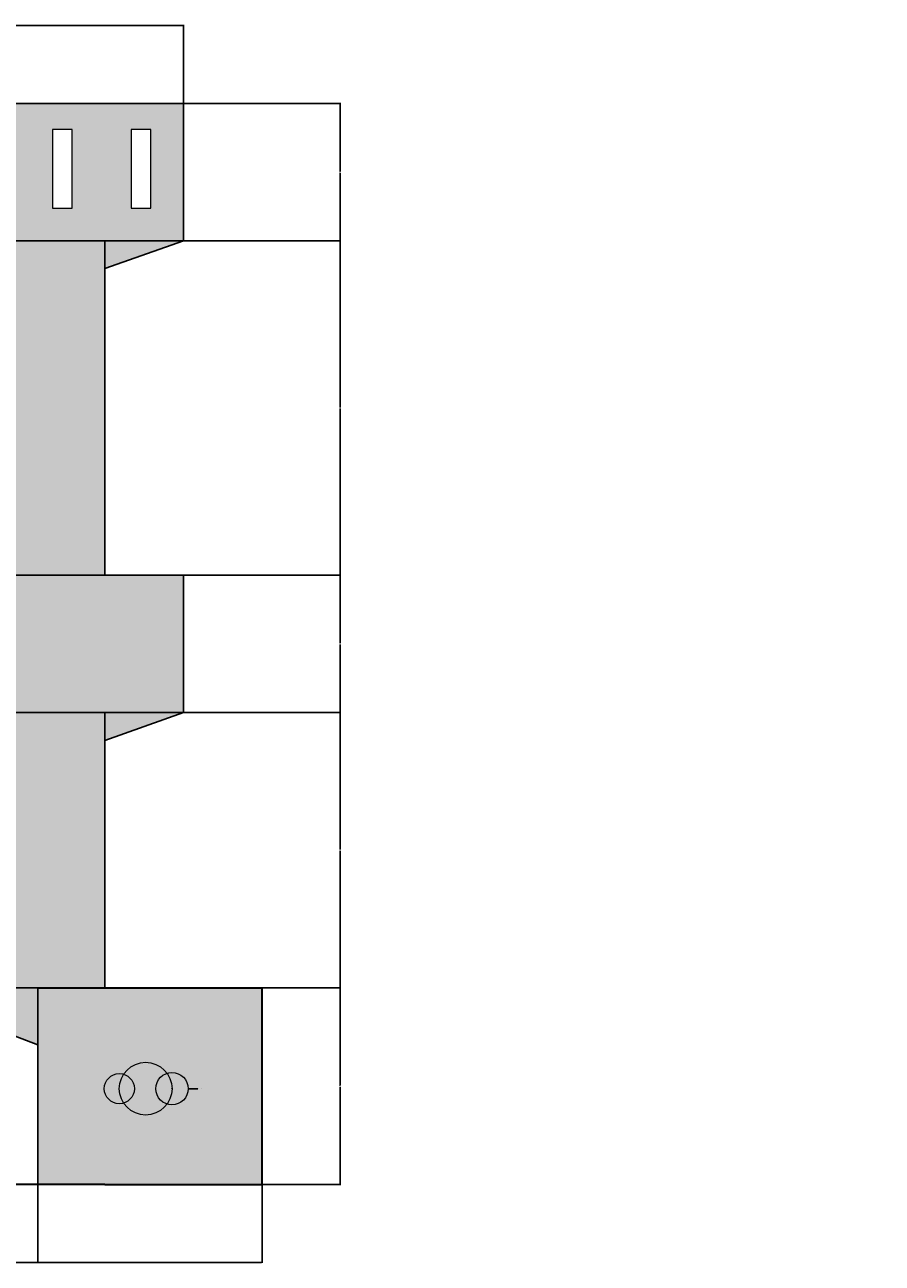
# Model space of a CAD drawing. Units: inches. Extents: x -43 to 1296, y -568 to 542.
# Tile 7 of 14: x 364 to 626, y 164 to 542. Entities that reach past the tile are written whole.
import ezdxf

# ---------------------------------------------------------------- set-up
doc = ezdxf.new("R2010")
doc.units = ezdxf.units.IN
doc.header["$MEASUREMENT"] = 0
for name, color, linetype, lineweight in [('A-ANNO-DIMS', 2, 'Continuous', 18), ('A-ELEV', 7, 'Continuous', 25), ('A-ELEV-TRIM', 7, 'Continuous', 18), ('A-ELEV-TRIM-PATT', 4, 'Continuous', 13), ('A-SITE-GATE', 7, 'Continuous', 25), ('A-SITE-WALL', 7, 'Continuous', 30), ('A-SITE-WALL-PATT', 142, 'Continuous', 13)]:
    doc.layers.add(name, color=color, linetype=linetype, lineweight=lineweight)
for name, color, linetype, lineweight, true_color in [('A-ELEV-BAND-PATT', 30, 'Continuous', 13, 0xf8991e), ('A-ELEV-WALL-PATT', 31, 'Continuous', 13, 0xfecc66), ('A-ROOF-PATT', 217, 'Continuous', 13, 0x93278f)]:
    doc.layers.add(name, color=color, linetype=linetype, lineweight=lineweight, true_color=true_color)
doc.styles.get("Standard").update_dxf_attribs({"font": 'arial.ttf'})
doc.dimstyles.get("Standard").update_dxf_attribs({"dimtxt": 0.18, "dimasz": 0.18, "dimexe": 0.18, "dimexo": 0.0625, "dimgap": 0.09, "dimtad": 0, "dimtih": 1, "dimtoh": 1, "dimdec": 0, "dimzin": 0, "dimdsep": 46, "dimlunit": 3, "dimtxsty": 'Standard', "dimcen": 0.09, "dimadec": 0, "dimazin": 0, "dimtfac": 1, "dimtdec": 0, "dimtofl": 0, "dimtmove": 0, "dimatfit": 3, "dimfxl": 1, "dimtolj": 1, "dimtzin": 0, "dimarcsym": 0})

# ---------------------------------------------------------------- blocks, each defined once
blk = doc.blocks.new('*U5')
for p, q in [((-3, 12), (-3, -12)), ((3, 12), (-3, 12)), ((3, -12), (3, 12)), ((-3, -12), (3, -12))]:
    blk.add_line(p, q)
blk = doc.blocks.new('*U6')
at = {"layer": 'A-ELEV-TRIM', "color": 0, "linetype": 'ByBlock', "lineweight": -2, "transparency": 16777216}
for p in [(0, 0), (24, 0), (48, 0), (72, 0), (96, 0), (120, 0), (144, 0), (168, 0), (192, 0), (216, 0), (240, 0), (264, 0), (288, 0), (312, 0), (336, 0), (360, 0), (384, 0)]:
    blk.add_blockref('*U5', p, dxfattribs=at)
blk = doc.blocks.new('*D60')
at = {"layer": 'A-ANNO-DIMS', "color": 0, "lineweight": -2, "transparency": 16777216}
for p, q in [((-19.16, 188.23), (-19.16, 164.31)), ((436.84, 188.23), (436.84, 164.31)), ((-18.98, 164.49), (208.44, 164.49)), ((436.66, 164.49), (209.24, 164.49))]:
    blk.add_line(p, q, dxfattribs=at)
at = {"layer": 'A-ANNO-DIMS', "color": 0, "transparency": 16777216}
for points in [[(-18.98, 164.52), (-18.98, 164.46), (-19.16, 164.49)], [(436.66, 164.52), (436.66, 164.46), (436.84, 164.49)]]:
    blk.add_solid(points, dxfattribs=at)
at = {"layer": 'Defpoints', "color": 0, "transparency": 16777216}
for p in [(-19.16, 188.29), (436.84, 188.29), (436.84, 164.49)]:
    blk.add_point(p, dxfattribs=at)
at = {"layer": 'A-ANNO-DIMS', "color": 0, "transparency": 16777216, "insert": (208.84, 164.49), "char_height": 0.18, "attachment_point": 5}
blk.add_mtext('\\A1;38\'-0"', dxfattribs=at)
blk = doc.blocks.new('*D62')
at = {"layer": 'A-ANNO-DIMS', "color": 0, "lineweight": -2, "transparency": 16777216}
for p, q in [((436.91, 248.29), (460.82, 248.29)), ((460.64, 248.11), (460.64, 218.47)), ((460.64, 188.47), (460.64, 218.11)), ((436.91, 188.29), (460.82, 188.29))]:
    blk.add_line(p, q, dxfattribs=at)
at = {"layer": 'A-ANNO-DIMS', "color": 0, "transparency": 16777216}
for points in [[(460.61, 248.11), (460.67, 248.11), (460.64, 248.29)], [(460.61, 188.47), (460.67, 188.47), (460.64, 188.29)]]:
    blk.add_solid(points, dxfattribs=at)
at = {"layer": 'Defpoints', "color": 0, "transparency": 16777216}
for p in [(436.84, 248.29), (460.64, 248.29), (436.84, 188.29)]:
    blk.add_point(p, dxfattribs=at)
at = {"layer": 'A-ANNO-DIMS', "color": 0, "transparency": 16777216, "insert": (460.64, 218.29), "char_height": 0.18, "attachment_point": 5}
blk.add_mtext('\\A1;5\'-0"', dxfattribs=at)
blk = doc.blocks.new('*D63')
at = {"layer": 'A-ANNO-DIMS', "color": 0, "lineweight": -2, "transparency": 16777216}
for p, q in [((412.91, 332.29), (460.82, 332.29)), ((460.64, 332.11), (460.64, 290.47)), ((460.64, 248.47), (460.64, 290.11)), ((436.91, 248.29), (460.82, 248.29))]:
    blk.add_line(p, q, dxfattribs=at)
at = {"layer": 'A-ANNO-DIMS', "color": 0, "transparency": 16777216}
for points in [[(460.61, 332.11), (460.67, 332.11), (460.64, 332.29)], [(460.61, 248.47), (460.67, 248.47), (460.64, 248.29)]]:
    blk.add_solid(points, dxfattribs=at)
at = {"layer": 'Defpoints', "color": 0, "transparency": 16777216}
for p in [(412.84, 332.29), (460.64, 332.29), (436.84, 248.29)]:
    blk.add_point(p, dxfattribs=at)
at = {"layer": 'A-ANNO-DIMS', "color": 0, "transparency": 16777216, "insert": (460.64, 290.29), "char_height": 0.18, "attachment_point": 5}
blk.add_mtext('\\A1;7\'-0"', dxfattribs=at)
blk = doc.blocks.new('*D64')
at = {"layer": 'A-ANNO-DIMS', "color": 0, "lineweight": -2, "transparency": 16777216}
for p, q in [((412.91, 374.29), (460.82, 374.29)), ((460.64, 374.11), (460.64, 353.47)), ((460.64, 332.47), (460.64, 353.11)), ((412.91, 332.29), (460.82, 332.29))]:
    blk.add_line(p, q, dxfattribs=at)
at = {"layer": 'A-ANNO-DIMS', "color": 0, "transparency": 16777216}
for points in [[(460.61, 374.11), (460.67, 374.11), (460.64, 374.29)], [(460.61, 332.47), (460.67, 332.47), (460.64, 332.29)]]:
    blk.add_solid(points, dxfattribs=at)
at = {"layer": 'Defpoints', "color": 0, "transparency": 16777216}
for p in [(412.84, 374.29), (460.64, 374.29), (412.84, 332.29)]:
    blk.add_point(p, dxfattribs=at)
at = {"layer": 'A-ANNO-DIMS', "color": 0, "transparency": 16777216, "insert": (460.64, 353.29), "char_height": 0.18, "attachment_point": 5}
blk.add_mtext('\\A1;3\'-6"', dxfattribs=at)
blk = doc.blocks.new('*D65')
at = {"layer": 'A-ANNO-DIMS', "color": 0, "lineweight": -2, "transparency": 16777216}
for p, q in [((412.91, 476.29), (460.82, 476.29)), ((460.64, 476.11), (460.64, 425.47)), ((460.64, 374.47), (460.64, 425.11)), ((412.91, 374.29), (460.82, 374.29))]:
    blk.add_line(p, q, dxfattribs=at)
at = {"layer": 'A-ANNO-DIMS', "color": 0, "transparency": 16777216}
for points in [[(460.61, 476.11), (460.67, 476.11), (460.64, 476.29)], [(460.61, 374.47), (460.67, 374.47), (460.64, 374.29)]]:
    blk.add_solid(points, dxfattribs=at)
at = {"layer": 'Defpoints', "color": 0, "transparency": 16777216}
for p in [(412.84, 476.29), (460.64, 476.29), (412.84, 374.29)]:
    blk.add_point(p, dxfattribs=at)
at = {"layer": 'A-ANNO-DIMS', "color": 0, "transparency": 16777216, "insert": (460.64, 425.29), "char_height": 0.18, "attachment_point": 5}
blk.add_mtext('\\A1;8\'-6"', dxfattribs=at)
blk = doc.blocks.new('*D66')
at = {"layer": 'A-ANNO-DIMS', "color": 0, "lineweight": -2, "transparency": 16777216}
for p, q in [((412.91, 518.29), (460.82, 518.29)), ((460.64, 518.11), (460.64, 497.47)), ((460.64, 476.47), (460.64, 497.11)), ((412.91, 476.29), (460.82, 476.29))]:
    blk.add_line(p, q, dxfattribs=at)
at = {"layer": 'A-ANNO-DIMS', "color": 0, "transparency": 16777216}
for points in [[(460.61, 518.11), (460.67, 518.11), (460.64, 518.29)], [(460.61, 476.47), (460.67, 476.47), (460.64, 476.29)]]:
    blk.add_solid(points, dxfattribs=at)
at = {"layer": 'Defpoints', "color": 0, "transparency": 16777216}
for p in [(412.84, 518.29), (460.64, 518.29), (412.84, 476.29)]:
    blk.add_point(p, dxfattribs=at)
at = {"layer": 'A-ANNO-DIMS', "color": 0, "transparency": 16777216, "insert": (460.64, 497.29), "char_height": 0.18, "attachment_point": 5}
blk.add_mtext('\\A1;3\'-6"', dxfattribs=at)
blk = doc.blocks.new('*D67')
at = {"layer": 'A-ANNO-DIMS', "color": 0, "lineweight": -2, "transparency": 16777216}
for p, q in [((277.84, 188.23), (277.84, 164.31)), ((368.43, 188.23), (368.43, 164.31)), ((278.02, 164.49), (322.6, 164.49)), ((368.25, 164.49), (323.68, 164.49))]:
    blk.add_line(p, q, dxfattribs=at)
at = {"layer": 'A-ANNO-DIMS', "color": 0, "transparency": 16777216}
for points in [[(278.02, 164.52), (278.02, 164.46), (277.84, 164.49)], [(368.25, 164.52), (368.25, 164.46), (368.43, 164.49)]]:
    blk.add_solid(points, dxfattribs=at)
at = {"layer": 'Defpoints', "color": 0, "transparency": 16777216}
for p in [(277.84, 188.29), (368.43, 188.29), (368.43, 164.49)]:
    blk.add_point(p, dxfattribs=at)
at = {"layer": 'A-ANNO-DIMS', "color": 0, "transparency": 16777216, "insert": (323.14, 164.49), "char_height": 0.18, "attachment_point": 5}
blk.add_mtext('\\A1;7\'-6 1/2"', dxfattribs=at)
blk = doc.blocks.new('*D69')
at = {"layer": 'A-ANNO-DIMS', "color": 0, "lineweight": -2, "transparency": 16777216}
for p, q in [((323.2, 248.29), (460.82, 248.29)), ((460.64, 248.11), (460.64, 218.47)), ((460.64, 188.47), (460.64, 218.11)), ((368.5, 188.29), (460.82, 188.29))]:
    blk.add_line(p, q, dxfattribs=at)
at = {"layer": 'A-ANNO-DIMS', "color": 0, "transparency": 16777216}
for points in [[(460.61, 248.11), (460.67, 248.11), (460.64, 248.29)], [(460.61, 188.47), (460.67, 188.47), (460.64, 188.29)]]:
    blk.add_solid(points, dxfattribs=at)
at = {"layer": 'Defpoints', "color": 0, "transparency": 16777216}
for p in [(323.14, 248.29), (368.43, 188.29), (460.64, 188.29)]:
    blk.add_point(p, dxfattribs=at)
at = {"layer": 'A-ANNO-DIMS', "color": 0, "transparency": 16777216, "insert": (460.64, 218.29), "char_height": 0.18, "attachment_point": 5}
blk.add_mtext('\\A1;5\'-0"', dxfattribs=at)
blk = doc.blocks.new('*D72')
at = {"layer": 'A-ANNO-DIMS', "color": 0, "lineweight": -2, "transparency": 16777216}
for p, q in [((368.43, 188.23), (368.43, 164.31)), ((436.84, 188.23), (436.84, 164.31)), ((368.61, 164.49), (402.1, 164.49)), ((436.66, 164.49), (403.18, 164.49))]:
    blk.add_line(p, q, dxfattribs=at)
at = {"layer": 'A-ANNO-DIMS', "color": 0, "transparency": 16777216}
for points in [[(368.61, 164.52), (368.61, 164.46), (368.43, 164.49)], [(436.66, 164.52), (436.66, 164.46), (436.84, 164.49)]]:
    blk.add_solid(points, dxfattribs=at)
at = {"layer": 'Defpoints', "color": 0, "transparency": 16777216}
for p in [(368.43, 188.29), (436.84, 188.29), (436.84, 164.49)]:
    blk.add_point(p, dxfattribs=at)
at = {"layer": 'A-ANNO-DIMS', "color": 0, "transparency": 16777216, "insert": (402.64, 164.49), "char_height": 0.18, "attachment_point": 5}
blk.add_mtext('\\A1;5\'-8 1/2"', dxfattribs=at)
blk = doc.blocks.new('*D73')
at = {"layer": 'A-ANNO-DIMS', "color": 0, "lineweight": -2, "transparency": 16777216}
for p, q in [((4.84, 518.35), (4.84, 542.27)), ((5.02, 542.09), (208.44, 542.09)), ((412.66, 542.09), (209.24, 542.09)), ((412.84, 518.35), (412.84, 542.27))]:
    blk.add_line(p, q, dxfattribs=at)
at = {"layer": 'A-ANNO-DIMS', "color": 0, "transparency": 16777216}
for points in [[(5.02, 542.12), (5.02, 542.06), (4.84, 542.09)], [(412.66, 542.12), (412.66, 542.06), (412.84, 542.09)]]:
    blk.add_solid(points, dxfattribs=at)
at = {"layer": 'Defpoints', "color": 0, "transparency": 16777216}
for p in [(412.84, 542.09), (4.84, 518.29), (412.84, 518.29)]:
    blk.add_point(p, dxfattribs=at)
at = {"layer": 'A-ANNO-DIMS', "color": 0, "transparency": 16777216, "insert": (208.84, 542.09), "char_height": 0.18, "attachment_point": 5}
blk.add_mtext('\\A1;34\'-0"', dxfattribs=at)
blk = doc.blocks.new('*D100')
at = {"layer": 'A-ANNO-DIMS', "color": 0, "lineweight": -2, "transparency": 16777216}
for p, q in [((409.23, 217.51), (409.41, 217.51)), ((409.32, 217.42), (409.32, 217.6)), ((417.2, 217.51), (414.42, 217.51))]:
    blk.add_line(p, q, dxfattribs=at)
at = {"layer": 'A-ANNO-DIMS', "color": 0, "transparency": 16777216}
blk.add_solid([(414.42, 217.54), (414.42, 217.48), (414.24, 217.51)], dxfattribs=at)
at = {"layer": 'Defpoints', "color": 0, "transparency": 16777216}
for p in [(404.4, 217.51), (414.24, 217.51)]:
    blk.add_point(p, dxfattribs=at)
at = {"layer": 'A-ANNO-DIMS', "color": 0, "transparency": 16777216, "insert": (417.88, 217.51), "char_height": 0.18, "attachment_point": 5}
blk.add_mtext('\\A1;3X ∅0\'-10"', dxfattribs=at)

msp = doc.modelspace()

# ---------------------------------------------------------------- hatches: boundary and pattern name
at = {"layer": 'A-ELEV-BAND-PATT'}
h = msp.add_hatch(color=256, dxfattribs=at)
h.dxf.hatch_style = 1
h.paths.add_polyline_path([(28.84, 332.29), (4.84, 332.29), (28.84, 320)])
h.paths.add_polyline_path([(412.84, 332.29), (388.84, 332.29), (388.84, 323.84)])
h.paths.add_polyline_path([(1184.13, 416.59), (824.13, 416.59), (824.13, 410.59), (1184.13, 410.59)])
h.paths.add_polyline_path([(1184.13, 272.59), (824.13, 272.59), (824.13, 266.59), (1184.13, 266.59)])
h = msp.add_hatch(color=256, dxfattribs=at)
h.dxf.hatch_style = 1
h.paths.add_polyline_path([(412.84, 374.29), (4.84, 374.29), (4.84, 332.29), (412.84, 332.29)])
h.paths.add_polyline_path([(222.28, 353.73, -0.197856), (210.28, 353.73, -0.131652), (209.89, 352.27, -0.197856), (220.28, 346.27, -0.197856), (209.89, 352.27, -0.131652), (208.82, 351.2, -0.197856), (214.82, 340.81, -0.197856), (208.82, 351.2, -0.131652), (207.36, 350.81, -0.197856), (207.36, 338.81, -0.197856), (207.36, 350.81, -0.131652), (205.9, 351.2, -0.197856), (199.9, 340.81, -0.197856), (205.9, 351.2, -0.131652), (204.83, 352.27, -0.197856), (194.44, 346.27, -0.197856), (204.83, 352.27, -0.131652), (204.44, 353.73, -0.197856), (192.44, 353.73, -0.197856), (204.44, 353.73, -0.131652), (204.83, 355.19, -0.197856), (194.44, 361.19, -0.197856), (204.83, 355.19, -0.131652), (205.9, 356.25, -0.197856), (199.9, 366.65, -0.197856), (205.9, 356.25, -0.131652), (207.36, 356.65, -0.197856), (207.36, 368.65, -0.197856), (207.36, 356.65, -0.131652), (208.82, 356.25, -0.197856), (214.82, 366.65, -0.197856), (208.82, 356.25, -0.131652), (209.89, 355.19, -0.197856), (220.28, 361.19, -0.197856), (209.89, 355.19, -0.131652), (210.28, 353.73, -0.197856)], flags=16)
h.paths.add_polyline_path([(263.61, 353.73, -0.197856), (275.61, 353.73, -0.131652), (276, 355.19, -0.197856), (265.61, 361.19, -0.197856), (276, 355.19, -0.131652), (277.07, 356.25, -0.197856), (271.07, 366.65, -0.197856), (277.07, 356.25, -0.131652), (278.53, 356.65, -0.197856), (278.53, 368.65, -0.197856), (278.53, 356.65, -0.131652), (279.99, 356.25, -0.197856), (285.99, 366.65, -0.197856), (279.99, 356.25, -0.131652), (281.06, 355.19, -0.197856), (291.45, 361.19, -0.197856), (281.06, 355.19, -0.131652), (281.45, 353.73, -0.197856), (293.45, 353.73, -0.197856), (281.45, 353.73, -0.131652), (281.06, 352.27, -0.197856), (291.45, 346.27, -0.197856), (281.06, 352.27, -0.131652), (279.99, 351.2, -0.197856), (285.99, 340.81, -0.197856), (279.99, 351.2, -0.131652), (278.53, 350.81, -0.197856), (278.53, 338.81, -0.197856), (278.53, 350.81, -0.131652), (277.07, 351.2, -0.197856), (271.07, 340.81, -0.197856), (277.07, 351.2, -0.131652), (276, 352.27, -0.197856), (265.61, 346.27, -0.197856), (276, 352.27, -0.131652), (275.61, 353.73, -0.197856)], flags=16)
h.paths.add_polyline_path([(330.52, 353.73, -0.197856), (342.52, 353.73, -0.131652), (342.91, 355.19, -0.197856), (332.52, 361.19, -0.197856), (342.91, 355.19, -0.131652), (343.98, 356.25, -0.197856), (337.98, 366.65, -0.197856), (343.98, 356.25, -0.131652), (345.44, 356.65, -0.197856), (345.44, 368.65, -0.197856), (345.44, 356.65, -0.131652), (346.9, 356.25, -0.197856), (352.9, 366.65, -0.197856), (346.9, 356.25, -0.131652), (347.97, 355.19, -0.197856), (358.36, 361.19, -0.197856), (347.97, 355.19, -0.131652), (348.36, 353.73, -0.197856), (360.36, 353.73, -0.197856), (348.36, 353.73, -0.131652), (347.97, 352.27, -0.197856), (358.36, 346.27, -0.197856), (347.97, 352.27, -0.131652), (346.9, 351.2, -0.197856), (352.9, 340.81, -0.197856), (346.9, 351.2, -0.131652), (345.44, 350.81, -0.197856), (345.44, 338.81, -0.197856), (345.44, 350.81, -0.131652), (343.98, 351.2, -0.197856), (337.98, 340.81, -0.197856), (343.98, 351.2, -0.131652), (342.91, 352.27, -0.197856), (332.52, 346.27, -0.197856), (342.91, 352.27, -0.131652), (342.52, 353.73, -0.197856)], flags=16)
h.paths.add_polyline_path([(148.25, 353.73, -0.197856), (136.25, 353.73, -0.131652), (135.85, 352.27, -0.197856), (146.25, 346.27, -0.197856), (135.85, 352.27, -0.131652), (134.79, 351.2, -0.197856), (140.79, 340.81, -0.197856), (134.79, 351.2, -0.131652), (133.33, 350.81, -0.197856), (133.33, 338.81, -0.197856), (133.33, 350.81, -0.131652), (131.87, 351.2, -0.197856), (125.87, 340.81, -0.197856), (131.87, 351.2, -0.131652), (130.8, 352.27, -0.197856), (120.41, 346.27, -0.197856), (130.8, 352.27, -0.131652), (130.41, 353.73, -0.197856), (118.41, 353.73, -0.197856), (130.41, 353.73, -0.131652), (130.8, 355.19, -0.197856), (120.41, 361.19, -0.197856), (130.8, 355.19, -0.131652), (131.87, 356.25, -0.197856), (125.87, 366.65, -0.197856), (131.87, 356.25, -0.131652), (133.33, 356.65, -0.197856), (133.33, 368.65, -0.197856), (133.33, 356.65, -0.131652), (134.79, 356.25, -0.197856), (140.79, 366.65, -0.197856), (134.79, 356.25, -0.131652), (135.85, 355.19, -0.197856), (146.25, 361.19, -0.197856), (135.85, 355.19, -0.131652), (136.25, 353.73, -0.197856)], flags=16)
h.paths.add_polyline_path([(80.61, 353.73, -0.197856), (68.61, 353.73, -0.131652), (68.22, 352.27, -0.197856), (78.61, 346.27, -0.197856), (68.22, 352.27, -0.131652), (67.15, 351.2, -0.197856), (73.15, 340.81, -0.197856), (67.15, 351.2, -0.131652), (65.69, 350.81, -0.197856), (65.69, 338.81, -0.197856), (65.69, 350.81, -0.131652), (64.23, 351.2, -0.197856), (58.23, 340.81, -0.197856), (64.23, 351.2, -0.131652), (63.16, 352.27, -0.197856), (52.77, 346.27, -0.197856), (63.16, 352.27, -0.131652), (62.77, 353.73, -0.197856), (50.77, 353.73, -0.197856), (62.77, 353.73, -0.131652), (63.16, 355.19, -0.197856), (52.77, 361.19, -0.197856), (63.16, 355.19, -0.131652), (64.23, 356.25, -0.197856), (58.23, 366.65, -0.197856), (64.23, 356.25, -0.131652), (65.69, 356.65, -0.197856), (65.69, 368.65, -0.197856), (65.69, 356.65, -0.131652), (67.15, 356.25, -0.197856), (73.15, 366.65, -0.197856), (67.15, 356.25, -0.131652), (68.22, 355.19, -0.197856), (78.61, 361.19, -0.197856), (68.22, 355.19, -0.131652), (68.61, 353.73, -0.197856)], flags=16)
at = {"layer": 'A-ELEV-TRIM-PATT'}
h = msp.add_hatch(color=256, dxfattribs=at)
h.dxf.hatch_style = 1
h.paths.add_polyline_path([(164.68, 212.9), (115.24, 229.23), (67.47, 212.06), (115.24, 194.9)])
h.paths.add_polyline_path([(116.88, 213.05, -0.289973), (115.08, 213.05, -0.198912), (114.88, 212.55, -0.289973), (116.15, 211.28, -0.289973), (114.88, 212.55, -0.198912), (114.38, 212.34, -0.289973), (114.38, 210.55, -0.289973), (114.38, 212.34, -0.198912), (113.88, 212.55, -0.289973), (112.61, 211.28, -0.289973), (113.88, 212.55, -0.198912), (113.68, 213.05, -0.289973), (111.88, 213.05, -0.289973), (113.68, 213.05, -0.198912), (113.88, 213.54, -0.289973), (112.61, 214.81, -0.289973), (113.88, 213.54, -0.198912), (114.38, 213.75, -0.289973), (114.38, 215.55, -0.289973), (114.38, 213.75, -0.198912), (114.88, 213.54, -0.289973), (116.15, 214.81, -0.289973), (114.88, 213.54, -0.198912), (115.08, 213.05, -0.289973)], flags=16)
h.paths.add_polyline_path([(218.46, 217.51, -0.325786), (221.87, 222.19, 0.526984), (208.61, 221.91, -0.331674), (211.89, 217.51, -0.331674), (208.61, 213.11, 0.526984), (221.87, 212.82, -0.325786)])
h.paths.add_polyline_path([(404.4, 217.51, -0.325786), (407.82, 222.19, 0.526984), (394.56, 221.91, -0.331674), (397.84, 217.51, -0.331674), (394.56, 213.11, 0.526984), (407.82, 212.82, -0.325786)])
h.paths.add_polyline_path([(14.67, 215.02, -0.325786), (18.08, 219.7, 0.526984), (4.82, 219.42, -0.331674), (8.11, 215.02, -0.331674), (4.82, 210.62, 0.526984), (18.08, 210.34, -0.325786)])
h = msp.add_hatch(color=256, dxfattribs=at)
h.dxf.hatch_style = 1
h.paths.add_polyline_path([(115.08, 213.05, 1), (113.68, 213.05, 1)])
h.paths.add_polyline_path([(114.38, 215.55, 0.289973), (114.38, 213.75, 0.289973)])
h.paths.add_polyline_path([(112.61, 214.81, 0.289973), (113.88, 213.54, 0.289973)])
h.paths.add_polyline_path([(113.68, 213.05, 0.289973), (111.88, 213.05, 0.289973)])
h.paths.add_polyline_path([(113.88, 212.55, 0.289973), (112.61, 211.28, 0.289973)])
h.paths.add_polyline_path([(114.38, 212.34, 0.289973), (114.38, 210.55, 0.289973)])
h.paths.add_polyline_path([(114.88, 212.55, 0.289973), (116.15, 211.28, 0.289973)])
h.paths.add_polyline_path([(115.08, 213.05, 0.289973), (116.88, 213.05, 0.289973)])
h.paths.add_polyline_path([(116.15, 214.81, 0.289973), (114.88, 213.54, 0.289973)])
h.paths.add_polyline_path([(8.11, 215.02, 0.331674), (4.82, 219.42, 0.145907), (3.51, 215.02, 0.145907), (4.82, 210.62, 0.331674)])
h.paths.add_polyline_path([(19.59, 215.02, 0.156779), (18.08, 219.7, 0.325786), (14.67, 215.02, 0.325786), (18.08, 210.34, 0.156779)])
h.paths.add_polyline_path([(18.08, 219.7, -0.156779), (19.59, 215.02, -0.156779), (18.08, 210.34, 0.508539), (24.51, 215.02, 0.508539)])
h.paths.add_polyline_path([(4.82, 219.42, 0.501869), (-1.08, 215.02, 0.501869), (4.82, 210.62, -0.145907), (3.51, 215.02, -0.145907)])
h.paths.add_polyline_path([(228.3, 217.51, 0.508539), (221.87, 222.19, -0.156779), (223.38, 217.51, -0.156779), (221.87, 212.82, 0.508539)])
h.paths.add_polyline_path([(223.38, 217.51, 0.156779), (221.87, 222.19, 0.325786), (218.46, 217.51, 0.325786), (221.87, 212.82, 0.156779)])
h.paths.add_polyline_path([(211.89, 217.51, 0.331674), (208.61, 221.91, 0.145907), (207.3, 217.51, 0.145907), (208.61, 213.11, 0.331674)])
h.paths.add_polyline_path([(208.61, 221.91, 0.501869), (202.71, 217.51, 0.501869), (208.61, 213.11, -0.145907), (207.3, 217.51, -0.145907)])
h.paths.add_polyline_path([(407.82, 222.19, -0.156779), (409.32, 217.51, -0.156779), (407.82, 212.82, 0.508539), (414.24, 217.51, 0.508539)])
h.paths.add_polyline_path([(393.25, 217.51, -0.145907), (394.56, 221.91, 0.501869), (388.65, 217.51, 0.501869), (394.56, 213.11, -0.145907)])
h.paths.add_polyline_path([(397.84, 217.51, 0.331674), (394.56, 221.91, 0.145907), (393.25, 217.51, 0.145907), (394.56, 213.11, 0.331674)])
h.paths.add_polyline_path([(409.32, 217.51, 0.156779), (407.82, 222.19, 0.325786), (404.4, 217.51, 0.325786), (407.82, 212.82, 0.156779)])
at = {"layer": 'A-ELEV-WALL-PATT'}
h = msp.add_hatch(color=256, dxfattribs=at)
h.dxf.hatch_style = 1
h.paths.add_polyline_path([(388.84, 476.29), (28.84, 476.29), (28.84, 374.29), (43.84, 374.29), (43.84, 434.29), (79.84, 434.29), (79.84, 374.29), (388.84, 374.29)])
h.paths.add_polyline_path([(123.34, 434.29), (183.34, 434.29), (183.34, 386.29), (123.34, 386.29)], flags=16)
h.paths.add_polyline_path([(277.84, 434.29), (337.84, 434.29), (337.84, 386.29), (277.84, 386.29)], flags=16)
h = msp.add_hatch(color=256, dxfattribs=at)
h.dxf.hatch_style = 1
h.paths.add_polyline_path([(388.84, 332.29), (28.84, 332.29), (28.84, 248.29), (43.84, 248.29), (43.84, 290.29), (79.84, 290.29), (79.84, 248.29), (123.34, 248.29), (123.34, 290.29), (183.34, 290.29), (183.34, 248.29), (277.84, 248.29), (277.84, 290.29), (337.84, 290.29), (337.84, 248.29), (337.84, 242.64), (368.43, 230.87), (368.43, 248.29), (388.84, 248.29)])
at = {"layer": 'A-ROOF-PATT'}
h = msp.add_hatch(color=256, dxfattribs=at)
h.dxf.hatch_style = 1
h.paths.add_polyline_path([(412.84, 518.29), (388.84, 518.29), (28.84, 518.29), (4.84, 518.29), (4.84, 476.29), (412.84, 476.29)])
h.paths.add_polyline_path([(204.9, 510.31), (210.9, 510.31), (210.9, 486.31), (204.9, 486.31)], flags=16)
h.paths.add_polyline_path([(186.9, 486.31), (180.9, 486.31), (180.9, 510.31), (186.9, 510.31)], flags=16)
h.paths.add_polyline_path([(228.9, 510.31), (234.9, 510.31), (234.9, 486.31), (228.9, 486.31)], flags=16)
h.paths.add_polyline_path([(162.9, 486.31), (156.9, 486.31), (156.9, 510.31), (162.9, 510.31)], flags=16)
h.paths.add_polyline_path([(252.9, 510.31), (258.9, 510.31), (258.9, 486.31), (252.9, 486.31)], flags=16)
h.paths.add_polyline_path([(138.9, 486.31), (132.9, 486.31), (132.9, 510.31), (138.9, 510.31)], flags=16)
h.paths.add_polyline_path([(276.9, 510.31), (282.9, 510.31), (282.9, 486.31), (276.9, 486.31)], flags=16)
h.paths.add_polyline_path([(114.9, 486.31), (108.9, 486.31), (108.9, 510.31), (114.9, 510.31)], flags=16)
h.paths.add_polyline_path([(300.9, 510.31), (306.9, 510.31), (306.9, 486.31), (300.9, 486.31)], flags=16)
h.paths.add_polyline_path([(90.9, 486.31), (84.9, 486.31), (84.9, 510.31), (90.9, 510.31)], flags=16)
h.paths.add_polyline_path([(324.9, 510.31), (330.9, 510.31), (330.9, 486.31), (324.9, 486.31)], flags=16)
h.paths.add_polyline_path([(66.9, 486.31), (60.9, 486.31), (60.9, 510.31), (66.9, 510.31)], flags=16)
h.paths.add_polyline_path([(348.9, 510.31), (354.9, 510.31), (354.9, 486.31), (348.9, 486.31)], flags=16)
h.paths.add_polyline_path([(42.9, 486.31), (36.9, 486.31), (36.9, 510.31), (42.9, 510.31)], flags=16)
h.paths.add_polyline_path([(372.9, 510.31), (378.9, 510.31), (378.9, 486.31), (372.9, 486.31)], flags=16)
h.paths.add_polyline_path([(18.9, 486.31), (12.9, 486.31), (12.9, 510.31), (18.9, 510.31)], flags=16)
h.paths.add_polyline_path([(396.9, 510.31), (402.9, 510.31), (402.9, 486.31), (396.9, 486.31)], flags=16)
h = msp.add_hatch(color=256, dxfattribs=at)
h.dxf.hatch_style = 1
h.paths.add_polyline_path([(28.84, 476.29), (4.84, 476.29), (28.84, 464)])
h.paths.add_polyline_path([(412.84, 476.29), (388.84, 476.29), (388.84, 467.84)])
at = {"layer": 'A-SITE-WALL-PATT'}
h = msp.add_hatch(color=256, dxfattribs=at)
h.dxf.hatch_style = 1
h.paths.add_polyline_path([(277.84, 248.29), (-19.16, 248.29), (-19.16, 188.29), (28.84, 188.29), (277.84, 188.29)])
h.paths.add_polyline_path([(115.24, 229.23), (164.68, 212.9), (115.24, 194.9), (67.47, 212.06)], flags=16)
h.paths.add_polyline_path([(112.61, 214.81, -0.289973), (113.88, 213.54, -0.198912), (114.38, 213.75, -0.289973), (114.38, 215.55, -0.289973), (114.38, 213.75, -0.198912), (114.88, 213.54, -0.289973), (116.15, 214.81, -0.289973), (114.88, 213.54, -0.198912), (115.08, 213.05, -0.289973), (116.88, 213.05, -0.289973), (115.08, 213.05, -0.198912), (114.88, 212.55, -0.289973), (116.15, 211.28, -0.289973), (114.88, 212.55, -0.198912), (114.38, 212.34, -0.289973), (114.38, 210.55, -0.289973), (114.38, 212.34, -0.198912), (113.88, 212.55, -0.289973), (112.61, 211.28, -0.289973), (113.88, 212.55, -0.198912), (113.68, 213.05, -0.289973), (111.88, 213.05, -0.289973), (113.68, 213.05, -0.198912), (113.88, 213.54, -0.289973)], flags=0)
h.paths.add_polyline_path([(24.51, 215.02, -0.508539), (18.08, 210.34, -0.526984), (4.82, 210.62, -0.501869), (-1.08, 215.02, -0.501869), (4.82, 219.42, -0.526984), (18.08, 219.7, -0.508539)], flags=16)
h.paths.add_polyline_path([(208.61, 221.91, -0.526984), (221.87, 222.19, -0.508539), (228.3, 217.51, -0.508539), (221.87, 212.82, -0.526984), (208.61, 213.11, -0.501869), (202.71, 217.51, -0.501869)], flags=16)
h.paths.add_polyline_path([(436.84, 248.29), (368.43, 248.29), (368.43, 188.29), (388.84, 188.29), (436.84, 188.29)])
h.paths.add_polyline_path([(394.56, 221.91, -0.526984), (407.82, 222.19, -0.508539), (414.24, 217.51, -0.508539), (407.82, 212.82, -0.526984), (394.56, 213.11, -0.501869), (388.65, 217.51, -0.501869)], flags=16)

# ---------------------------------------------------------------- linework, layer by layer
at = {"layer": 'A-ELEV'}
for p, q in [((388.84, 518.29), (28.84, 518.29)), ((412.84, 518.29), (388.84, 518.29)), ((412.84, 476.29), (412.84, 518.29)), ((412.84, 476.29), (4.84, 476.29)), ((388.84, 374.29), (388.84, 476.29)), ((412.84, 476.29), (388.84, 467.84)), ((412.84, 374.29), (4.84, 374.29)), ((412.84, 332.29), (412.84, 374.29)), ((412.84, 332.29), (4.84, 332.29)), ((388.84, 248.29), (388.84, 332.29)), ((412.84, 332.29), (388.84, 323.84))]:
    msp.add_line(p, q, dxfattribs=at)
at = {"layer": 'A-ELEV-TRIM'}
for centre, radius in [((401.29, 217.51), 8.04), ((393.25, 217.51), 4.59), ((409.32, 217.51), 4.92)]:
    msp.add_circle(centre, radius, dxfattribs=at)
at = {"layer": 'A-SITE-GATE'}
for p, q in [((323.14, 248.29), (368.43, 230.87)), ((368.43, 248.29), (368.43, 188.29))]:
    msp.add_line(p, q, dxfattribs=at)
at = {"layer": 'A-SITE-WALL'}
for p, q in [((368.43, 248.29), (436.84, 248.29)), ((436.84, 188.29), (436.84, 248.29)), ((388.84, 188.29), (28.84, 188.29)), ((388.84, 188.29), (436.84, 188.29))]:
    msp.add_line(p, q, dxfattribs=at)

# ---------------------------------------------------------------- block references
at = {"layer": 'A-ELEV-TRIM'}
msp.add_blockref('*U6', (15.9, 498.31), dxfattribs=at)

# ---------------------------------------------------------------- dimensions: what is measured, and where the dimension line sits
at = {"layer": 'A-ANNO-DIMS'}
for base, p1, p2, picture, middle in [((412.84, 542.09), (4.84, 518.29), (412.84, 518.29), '*D73', (208.84, 542.09)), ((436.84, 164.49), (-19.16, 188.29), (436.84, 188.29), '*D60', (208.84, 164.49)), ((368.43, 164.49), (277.84, 188.29), (368.43, 188.29), '*D67', (323.14, 164.49)), ((436.84, 164.49), (368.43, 188.29), (436.84, 188.29), '*D72', (402.64, 164.49))]:
    dim = msp.add_linear_dim(base=base, p1=p1, p2=p2, dimstyle='Standard', override={"dimdec": 1, "dimlfac": 1, "dimrnd": 0, "dimzin": 1, "dimdsep": 46, "dimlunit": 4, "dimfrac": 2}, dxfattribs=at)
    dim.commit()
    dim.dimension.update_dxf_attribs({"geometry": picture, "text_midpoint": middle})
for base, p1, p2, picture, middle in [((460.64, 518.29), (412.84, 476.29), (412.84, 518.29), '*D66', (460.64, 497.29)), ((460.64, 476.29), (412.84, 374.29), (412.84, 476.29), '*D65', (460.64, 425.29)), ((460.64, 374.29), (412.84, 332.29), (412.84, 374.29), '*D64', (460.64, 353.29)), ((460.64, 332.29), (436.84, 248.29), (412.84, 332.29), '*D63', (460.64, 290.29)), ((460.64, 188.29), (323.14, 248.29), (368.43, 188.29), '*D69', (460.64, 218.29)), ((460.64, 248.29), (436.84, 188.29), (436.84, 248.29), '*D62', (460.64, 218.29))]:
    dim = msp.add_linear_dim(base=base, p1=p1, p2=p2, angle=90, dimstyle='Standard', override={"dimdec": 1, "dimlfac": 1, "dimrnd": 0, "dimzin": 1, "dimdsep": 46, "dimlunit": 4, "dimfrac": 2}, dxfattribs=at)
    dim.commit()
    dim.dimension.update_dxf_attribs({"geometry": picture, "text_midpoint": middle})
dim = msp.add_diameter_dim_2p(p1=(404.4, 217.51), p2=(414.24, 217.51), text='3X <>', dimstyle='Standard', override={"dimdec": 1, "dimlfac": 1, "dimrnd": 0, "dimzin": 1, "dimdsep": 46, "dimlunit": 4, "dimfrac": 2}, dxfattribs=at)
dim.commit()
dim.dimension.update_dxf_attribs({"geometry": '*D100', "text_midpoint": (417.2, 217.51), "dimtype": 163})

doc.saveas('drawing.dxf')
